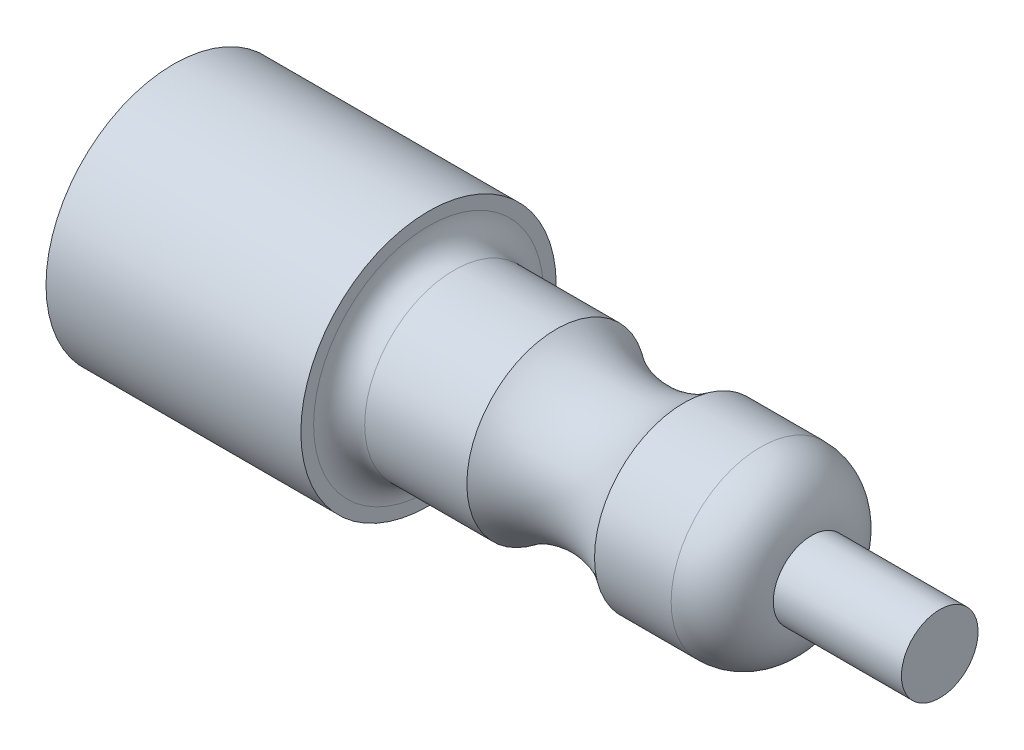
ISO-10303-21;
HEADER;
FILE_DESCRIPTION(('STEP AP214'),'2;1');
FILE_NAME('part.step','',(''),(''),'','','');
FILE_SCHEMA(('AUTOMOTIVE_DESIGN { 1 0 10303 214 1 1 1 1 }'));
ENDSEC;
DATA;
#1=APPLICATION_CONTEXT('core data for automotive mechanical design processes');
#2=APPLICATION_PROTOCOL_DEFINITION('international standard','automotive_design',2000,#1);
#3=PRODUCT_CONTEXT('',#1,'mechanical');
#4=PRODUCT('Part','Part','',(#3));
#5=PRODUCT_RELATED_PRODUCT_CATEGORY('part','',(#4));
#6=PRODUCT_DEFINITION_FORMATION('','',#4);
#7=PRODUCT_DEFINITION_CONTEXT('part definition',#1,'design');
#8=PRODUCT_DEFINITION('design','',#6,#7);
#9=PRODUCT_DEFINITION_SHAPE('','',#8);
#10=(LENGTH_UNIT() NAMED_UNIT(*) SI_UNIT(.MILLI.,.METRE.));
#11=(NAMED_UNIT(*) PLANE_ANGLE_UNIT() SI_UNIT($,.RADIAN.));
#12=(NAMED_UNIT(*) SI_UNIT($,.STERADIAN.) SOLID_ANGLE_UNIT());
#13=UNCERTAINTY_MEASURE_WITH_UNIT(LENGTH_MEASURE(1.E-05),#10,'distance_accuracy_value','');
#14=(GEOMETRIC_REPRESENTATION_CONTEXT(3) GLOBAL_UNCERTAINTY_ASSIGNED_CONTEXT((#13)) GLOBAL_UNIT_ASSIGNED_CONTEXT((#10,
#11,#12)) REPRESENTATION_CONTEXT('',''));
#15=CARTESIAN_POINT('',(0.,0.,0.));
#16=DIRECTION('',(0.,0.,1.));
#17=DIRECTION('',(1.,0.,0.));
#18=AXIS2_PLACEMENT_3D('',#15,#16,#17);
#19=CARTESIAN_POINT('',(0.,-0.5,0.));
#20=DIRECTION('',(-1.,0.,0.));
#21=DIRECTION('',(0.,0.,1.));
#22=AXIS2_PLACEMENT_3D('',#19,#20,#21);
#23=PLANE('',#22);
#24=CARTESIAN_POINT('',(0.,0.,0.));
#25=DIRECTION('',(-1.,0.,0.));
#26=DIRECTION('',(0.,0.,1.));
#27=AXIS2_PLACEMENT_3D('',#24,#25,#26);
#28=CIRCLE('',#27,0.5);
#29=CARTESIAN_POINT('',(0.,0.,0.5));
#30=VERTEX_POINT('',#29);
#31=EDGE_CURVE('E10',#30,#30,#28,.T.);
#32=ORIENTED_EDGE('',*,*,#31,.T.);
#33=EDGE_LOOP('',(#32));
#34=FACE_BOUND('',#33,.T.);
#35=ADVANCED_FACE('F40',(#34),#23,.T.);
#36=CARTESIAN_POINT('',(0.,0.,0.));
#37=DIRECTION('',(-1.,0.,0.));
#38=DIRECTION('',(0.,0.,1.));
#39=AXIS2_PLACEMENT_3D('',#36,#37,#38);
#40=CYLINDRICAL_SURFACE('',#39,0.5);
#41=CARTESIAN_POINT('',(0.998017857775598,0.,0.));
#42=DIRECTION('',(-1.,0.,0.));
#43=DIRECTION('',(0.,0.,1.));
#44=AXIS2_PLACEMENT_3D('',#41,#42,#43);
#45=CIRCLE('',#44,0.5);
#46=CARTESIAN_POINT('',(0.998017857775598,0.,0.5));
#47=VERTEX_POINT('',#46);
#48=EDGE_CURVE('E43',#47,#47,#45,.T.);
#49=ORIENTED_EDGE('',*,*,#48,.T.);
#50=EDGE_LOOP('',(#49));
#51=FACE_BOUND('',#50,.T.);
#52=ORIENTED_EDGE('',*,*,#31,.F.);
#53=EDGE_LOOP('',(#52));
#54=FACE_BOUND('',#53,.T.);
#55=ADVANCED_FACE('F84',(#51,#54),#40,.T.);
#56=CARTESIAN_POINT('',(0.998017857775598,-0.450000000000001,0.));
#57=DIRECTION('',(1.,0.,0.));
#58=DIRECTION('',(0.,0.,-1.));
#59=AXIS2_PLACEMENT_3D('',#56,#57,#58);
#60=PLANE('',#59);
#61=CARTESIAN_POINT('',(0.998017857775598,0.,0.));
#62=DIRECTION('',(-1.,0.,0.));
#63=DIRECTION('',(0.,0.,1.));
#64=AXIS2_PLACEMENT_3D('',#61,#62,#63);
#65=CIRCLE('',#64,0.450000000000001);
#66=CARTESIAN_POINT('',(0.998017857775598,0.,0.450000000000001));
#67=VERTEX_POINT('',#66);
#68=EDGE_CURVE('E50',#67,#67,#65,.T.);
#69=ORIENTED_EDGE('',*,*,#68,.T.);
#70=EDGE_LOOP('',(#69));
#71=FACE_BOUND('',#70,.T.);
#72=ORIENTED_EDGE('',*,*,#48,.F.);
#73=EDGE_LOOP('',(#72));
#74=FACE_BOUND('',#73,.T.);
#75=ADVANCED_FACE('F88',(#71,#74),#60,.T.);
#76=CARTESIAN_POINT('',(1.0980178577756,0.,0.));
#77=DIRECTION('',(-1.,0.,0.));
#78=DIRECTION('',(0.,0.,1.));
#79=AXIS2_PLACEMENT_3D('',#76,#77,#78);
#80=TOROIDAL_SURFACE('',#79,0.45,0.1);
#81=CARTESIAN_POINT('',(1.0980178577756,0.,0.));
#82=DIRECTION('',(-1.,0.,0.));
#83=DIRECTION('',(0.,0.,1.));
#84=AXIS2_PLACEMENT_3D('',#81,#82,#83);
#85=CIRCLE('',#84,0.35);
#86=CARTESIAN_POINT('',(1.0980178577756,0.,0.35));
#87=VERTEX_POINT('',#86);
#88=EDGE_CURVE('E51',#87,#87,#85,.T.);
#89=ORIENTED_EDGE('',*,*,#88,.T.);
#90=EDGE_LOOP('',(#89));
#91=FACE_BOUND('',#90,.T.);
#92=ORIENTED_EDGE('',*,*,#68,.F.);
#93=EDGE_LOOP('',(#92));
#94=FACE_BOUND('',#93,.T.);
#95=ADVANCED_FACE('F95',(#91,#94),#80,.F.);
#96=CARTESIAN_POINT('',(0.,0.,0.));
#97=DIRECTION('',(-1.,0.,0.));
#98=DIRECTION('',(0.,0.,1.));
#99=AXIS2_PLACEMENT_3D('',#96,#97,#98);
#100=CYLINDRICAL_SURFACE('',#99,0.35);
#101=CARTESIAN_POINT('',(1.4980178577756,0.,0.));
#102=DIRECTION('',(-1.,0.,0.));
#103=DIRECTION('',(0.,0.,1.));
#104=AXIS2_PLACEMENT_3D('',#101,#102,#103);
#105=CIRCLE('',#104,0.35);
#106=CARTESIAN_POINT('',(1.4980178577756,0.,0.35));
#107=VERTEX_POINT('',#106);
#108=EDGE_CURVE('E57',#107,#107,#105,.T.);
#109=ORIENTED_EDGE('',*,*,#108,.T.);
#110=EDGE_LOOP('',(#109));
#111=FACE_BOUND('',#110,.T.);
#112=ORIENTED_EDGE('',*,*,#88,.F.);
#113=EDGE_LOOP('',(#112));
#114=FACE_BOUND('',#113,.T.);
#115=ADVANCED_FACE('F98',(#111,#114),#100,.T.);
#116=CARTESIAN_POINT('',(1.7480178577756,0.,0.));
#117=DIRECTION('',(-1.,0.,0.));
#118=DIRECTION('',(0.,0.,1.));
#119=AXIS2_PLACEMENT_3D('',#116,#117,#118);
#120=TOROIDAL_SURFACE('',#119,0.681247641501038,0.415);
#121=CARTESIAN_POINT('',(1.9980178577756,0.,0.));
#122=DIRECTION('',(-1.,0.,0.));
#123=DIRECTION('',(0.,0.,1.));
#124=AXIS2_PLACEMENT_3D('',#121,#122,#123);
#125=CIRCLE('',#124,0.35);
#126=CARTESIAN_POINT('',(1.9980178577756,0.,0.35));
#127=VERTEX_POINT('',#126);
#128=EDGE_CURVE('E56',#127,#127,#125,.T.);
#129=ORIENTED_EDGE('',*,*,#128,.T.);
#130=EDGE_LOOP('',(#129));
#131=FACE_BOUND('',#130,.T.);
#132=ORIENTED_EDGE('',*,*,#108,.F.);
#133=EDGE_LOOP('',(#132));
#134=FACE_BOUND('',#133,.T.);
#135=ADVANCED_FACE('F104',(#131,#134),#120,.F.);
#136=CARTESIAN_POINT('',(0.,0.,0.));
#137=DIRECTION('',(-1.,0.,0.));
#138=DIRECTION('',(0.,0.,1.));
#139=AXIS2_PLACEMENT_3D('',#136,#137,#138);
#140=CYLINDRICAL_SURFACE('',#139,0.35);
#141=CARTESIAN_POINT('',(2.2980178577756,0.,0.));
#142=DIRECTION('',(-1.,0.,0.));
#143=DIRECTION('',(0.,0.,1.));
#144=AXIS2_PLACEMENT_3D('',#141,#142,#143);
#145=CIRCLE('',#144,0.35);
#146=CARTESIAN_POINT('',(2.2980178577756,0.,0.35));
#147=VERTEX_POINT('',#146);
#148=EDGE_CURVE('E65',#147,#147,#145,.T.);
#149=ORIENTED_EDGE('',*,*,#148,.T.);
#150=EDGE_LOOP('',(#149));
#151=FACE_BOUND('',#150,.T.);
#152=ORIENTED_EDGE('',*,*,#128,.F.);
#153=EDGE_LOOP('',(#152));
#154=FACE_BOUND('',#153,.T.);
#155=ADVANCED_FACE('F110',(#151,#154),#140,.T.);
#156=CARTESIAN_POINT('',(2.2980178577756,0.,0.));
#157=DIRECTION('',(-1.,0.,0.));
#158=DIRECTION('',(0.,0.,1.));
#159=AXIS2_PLACEMENT_3D('',#156,#157,#158);
#160=DEGENERATE_TOROIDAL_SURFACE('',#159,0.15,0.2,.T.);
#161=CARTESIAN_POINT('',(2.4980178577756,0.,0.));
#162=DIRECTION('',(-1.,0.,0.));
#163=DIRECTION('',(0.,0.,1.));
#164=AXIS2_PLACEMENT_3D('',#161,#162,#163);
#165=CIRCLE('',#164,0.15);
#166=CARTESIAN_POINT('',(2.4980178577756,0.,0.15));
#167=VERTEX_POINT('',#166);
#168=EDGE_CURVE('E61',#167,#167,#165,.T.);
#169=ORIENTED_EDGE('',*,*,#168,.T.);
#170=EDGE_LOOP('',(#169));
#171=FACE_BOUND('',#170,.T.);
#172=ORIENTED_EDGE('',*,*,#148,.F.);
#173=EDGE_LOOP('',(#172));
#174=FACE_BOUND('',#173,.T.);
#175=ADVANCED_FACE('F83',(#171,#174),#160,.T.);
#176=CARTESIAN_POINT('',(0.,0.,0.));
#177=DIRECTION('',(-1.,0.,0.));
#178=DIRECTION('',(0.,0.,1.));
#179=AXIS2_PLACEMENT_3D('',#176,#177,#178);
#180=CYLINDRICAL_SURFACE('',#179,0.15);
#181=CARTESIAN_POINT('',(3.,0.,0.));
#182=DIRECTION('',(-1.,0.,0.));
#183=DIRECTION('',(0.,0.,1.));
#184=AXIS2_PLACEMENT_3D('',#181,#182,#183);
#185=CIRCLE('',#184,0.15);
#186=CARTESIAN_POINT('',(3.,0.,0.15));
#187=VERTEX_POINT('',#186);
#188=EDGE_CURVE('E66',#187,#187,#185,.T.);
#189=ORIENTED_EDGE('',*,*,#188,.T.);
#190=EDGE_LOOP('',(#189));
#191=FACE_BOUND('',#190,.T.);
#192=ORIENTED_EDGE('',*,*,#168,.F.);
#193=EDGE_LOOP('',(#192));
#194=FACE_BOUND('',#193,.T.);
#195=ADVANCED_FACE('F75',(#191,#194),#180,.T.);
#196=CARTESIAN_POINT('',(3.,0.,0.));
#197=DIRECTION('',(1.,0.,0.));
#198=DIRECTION('',(0.,0.,-1.));
#199=AXIS2_PLACEMENT_3D('',#196,#197,#198);
#200=PLANE('',#199);
#201=ORIENTED_EDGE('',*,*,#188,.F.);
#202=EDGE_LOOP('',(#201));
#203=FACE_BOUND('',#202,.T.);
#204=ADVANCED_FACE('F71',(#203),#200,.T.);
#205=CLOSED_SHELL('',(#35,#55,#75,#95,#115,#135,#155,#175,#195,#204));
#206=MANIFOLD_SOLID_BREP('B2',#205);
#207=ADVANCED_BREP_SHAPE_REPRESENTATION('',(#18,#206),#14);
#208=SHAPE_DEFINITION_REPRESENTATION(#9,#207);
ENDSEC;
END-ISO-10303-21;
